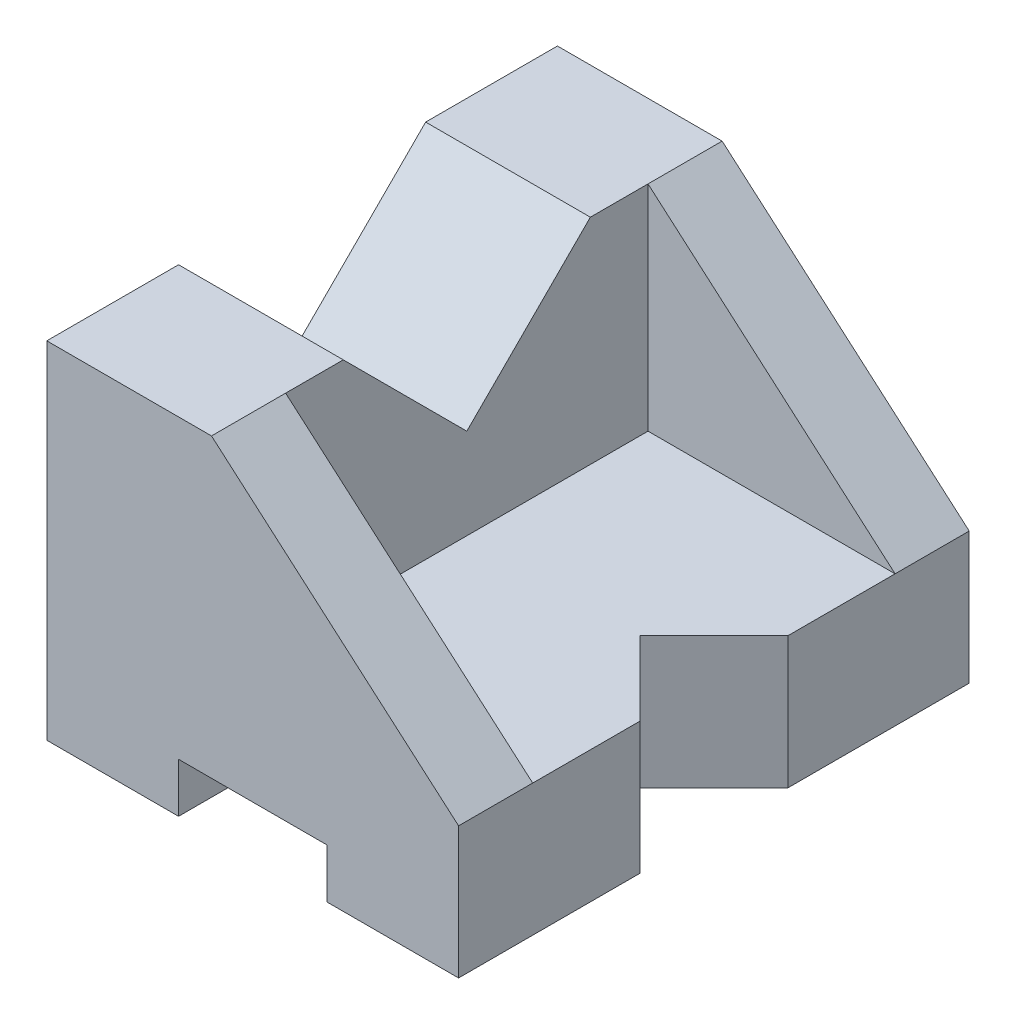
ISO-10303-21;
HEADER;
FILE_DESCRIPTION(('STEP AP214'),'2;1');
FILE_NAME('part.step','',(''),(''),'','','');
FILE_SCHEMA(('AUTOMOTIVE_DESIGN { 1 0 10303 214 1 1 1 1 }'));
ENDSEC;
DATA;
#1=APPLICATION_CONTEXT('core data for automotive mechanical design processes');
#2=APPLICATION_PROTOCOL_DEFINITION('international standard','automotive_design',2000,#1);
#3=PRODUCT_CONTEXT('',#1,'mechanical');
#4=PRODUCT('Part','Part','',(#3));
#5=PRODUCT_RELATED_PRODUCT_CATEGORY('part','',(#4));
#6=PRODUCT_DEFINITION_FORMATION('','',#4);
#7=PRODUCT_DEFINITION_CONTEXT('part definition',#1,'design');
#8=PRODUCT_DEFINITION('design','',#6,#7);
#9=PRODUCT_DEFINITION_SHAPE('','',#8);
#10=(LENGTH_UNIT() NAMED_UNIT(*) SI_UNIT(.MILLI.,.METRE.));
#11=(NAMED_UNIT(*) PLANE_ANGLE_UNIT() SI_UNIT($,.RADIAN.));
#12=(NAMED_UNIT(*) SI_UNIT($,.STERADIAN.) SOLID_ANGLE_UNIT());
#13=UNCERTAINTY_MEASURE_WITH_UNIT(LENGTH_MEASURE(1.E-05),#10,'distance_accuracy_value','');
#14=(GEOMETRIC_REPRESENTATION_CONTEXT(3) GLOBAL_UNCERTAINTY_ASSIGNED_CONTEXT((#13)) GLOBAL_UNIT_ASSIGNED_CONTEXT((#10,
#11,#12)) REPRESENTATION_CONTEXT('',''));
#15=CARTESIAN_POINT('',(0.,0.,0.));
#16=DIRECTION('',(0.,0.,1.));
#17=DIRECTION('',(1.,0.,0.));
#18=AXIS2_PLACEMENT_3D('',#15,#16,#17);
#19=CARTESIAN_POINT('',(-50.,0.,62.));
#20=DIRECTION('',(0.,1.,0.));
#21=DIRECTION('',(0.,0.,1.));
#22=AXIS2_PLACEMENT_3D('',#19,#20,#21);
#23=PLANE('',#22);
#24=DIRECTION('',(0.,0.,1.));
#25=VECTOR('',#24,1.);
#26=CARTESIAN_POINT('',(18.,0.,-62.001));
#27=LINE('',#26,#25);
#28=CARTESIAN_POINT('',(18.,0.,-62.));
#29=VERTEX_POINT('',#28);
#30=CARTESIAN_POINT('',(18.,0.,62.));
#31=VERTEX_POINT('',#30);
#32=EDGE_CURVE('E166',#29,#31,#27,.T.);
#33=ORIENTED_EDGE('',*,*,#32,.F.);
#34=DIRECTION('',(1.,0.,0.));
#35=VECTOR('',#34,1.);
#36=CARTESIAN_POINT('',(-50.,0.,-62.));
#37=LINE('',#36,#35);
#38=CARTESIAN_POINT('',(50.,0.,-62.));
#39=VERTEX_POINT('',#38);
#40=EDGE_CURVE('E190',#29,#39,#37,.T.);
#41=ORIENTED_EDGE('',*,*,#40,.T.);
#42=DIRECTION('',(0.,0.,-1.));
#43=VECTOR('',#42,1.);
#44=CARTESIAN_POINT('',(50.,0.,62.));
#45=LINE('',#44,#43);
#46=CARTESIAN_POINT('',(50.,0.,-18.));
#47=VERTEX_POINT('',#46);
#48=EDGE_CURVE('E216',#47,#39,#45,.T.);
#49=ORIENTED_EDGE('',*,*,#48,.F.);
#50=DIRECTION('',(0.707106781186548,0.,-0.707106781186547));
#51=VECTOR('',#50,1.);
#52=CARTESIAN_POINT('',(50.,0.,-18.));
#53=LINE('',#52,#51);
#54=CARTESIAN_POINT('',(32.,0.,0.));
#55=VERTEX_POINT('',#54);
#56=EDGE_CURVE('E297',#55,#47,#53,.T.);
#57=ORIENTED_EDGE('',*,*,#56,.F.);
#58=DIRECTION('',(-0.707106781186548,0.,-0.707106781186547));
#59=VECTOR('',#58,1.);
#60=CARTESIAN_POINT('',(32.,0.,0.));
#61=LINE('',#60,#59);
#62=CARTESIAN_POINT('',(50.,0.,18.));
#63=VERTEX_POINT('',#62);
#64=EDGE_CURVE('E312',#63,#55,#61,.T.);
#65=ORIENTED_EDGE('',*,*,#64,.F.);
#66=CARTESIAN_POINT('',(50.,0.,62.));
#67=VERTEX_POINT('',#66);
#68=EDGE_CURVE('E220',#67,#63,#45,.T.);
#69=ORIENTED_EDGE('',*,*,#68,.F.);
#70=DIRECTION('',(1.,0.,0.));
#71=VECTOR('',#70,1.);
#72=CARTESIAN_POINT('',(-50.,0.,62.));
#73=LINE('',#72,#71);
#74=EDGE_CURVE('E267',#31,#67,#73,.T.);
#75=ORIENTED_EDGE('',*,*,#74,.F.);
#76=EDGE_LOOP('',(#33,#41,#49,#57,#65,#69,#75));
#77=FACE_BOUND('',#76,.T.);
#78=ADVANCED_FACE('F39',(#77),#23,.F.);
#79=CARTESIAN_POINT('',(0.,0.,-62.));
#80=DIRECTION('',(0.,0.,1.));
#81=DIRECTION('',(1.,0.,0.));
#82=AXIS2_PLACEMENT_3D('',#79,#80,#81);
#83=PLANE('',#82);
#84=DIRECTION('',(0.,1.,0.));
#85=VECTOR('',#84,1.);
#86=CARTESIAN_POINT('',(-18.,0.,-62.));
#87=LINE('',#86,#85);
#88=CARTESIAN_POINT('',(-18.,0.,-62.));
#89=VERTEX_POINT('',#88);
#90=CARTESIAN_POINT('',(-18.,12.,-62.));
#91=VERTEX_POINT('',#90);
#92=EDGE_CURVE('E53',#89,#91,#87,.T.);
#93=ORIENTED_EDGE('',*,*,#92,.F.);
#94=CARTESIAN_POINT('',(-50.,0.,-62.));
#95=VERTEX_POINT('',#94);
#96=EDGE_CURVE('E177',#95,#89,#37,.T.);
#97=ORIENTED_EDGE('',*,*,#96,.F.);
#98=DIRECTION('',(0.,-1.,0.));
#99=VECTOR('',#98,1.);
#100=CARTESIAN_POINT('',(-50.,84.,-62.));
#101=LINE('',#100,#99);
#102=CARTESIAN_POINT('',(-50.,84.,-62.));
#103=VERTEX_POINT('',#102);
#104=EDGE_CURVE('E195',#103,#95,#101,.T.);
#105=ORIENTED_EDGE('',*,*,#104,.F.);
#106=DIRECTION('',(-1.,0.,0.));
#107=VECTOR('',#106,1.);
#108=CARTESIAN_POINT('',(-10.,84.,-62.));
#109=LINE('',#108,#107);
#110=CARTESIAN_POINT('',(-10.,84.,-62.));
#111=VERTEX_POINT('',#110);
#112=EDGE_CURVE('E196',#111,#103,#109,.T.);
#113=ORIENTED_EDGE('',*,*,#112,.F.);
#114=DIRECTION('',(-0.755689082789818,0.654930538417842,0.));
#115=VECTOR('',#114,1.);
#116=CARTESIAN_POINT('',(50.,32.,-62.));
#117=LINE('',#116,#115);
#118=CARTESIAN_POINT('',(50.,32.,-62.));
#119=VERTEX_POINT('',#118);
#120=EDGE_CURVE('E187',#119,#111,#117,.T.);
#121=ORIENTED_EDGE('',*,*,#120,.F.);
#122=DIRECTION('',(0.,1.,0.));
#123=VECTOR('',#122,1.);
#124=CARTESIAN_POINT('',(50.,0.,-62.));
#125=LINE('',#124,#123);
#126=EDGE_CURVE('E188',#39,#119,#125,.T.);
#127=ORIENTED_EDGE('',*,*,#126,.F.);
#128=ORIENTED_EDGE('',*,*,#40,.F.);
#129=DIRECTION('',(0.,-1.,0.));
#130=VECTOR('',#129,1.);
#131=CARTESIAN_POINT('',(18.,0.,-62.));
#132=LINE('',#131,#130);
#133=CARTESIAN_POINT('',(18.,12.,-62.));
#134=VERTEX_POINT('',#133);
#135=EDGE_CURVE('E305',#134,#29,#132,.T.);
#136=ORIENTED_EDGE('',*,*,#135,.F.);
#137=DIRECTION('',(1.,0.,0.));
#138=VECTOR('',#137,1.);
#139=CARTESIAN_POINT('',(-18.,12.,-62.));
#140=LINE('',#139,#138);
#141=EDGE_CURVE('E178',#91,#134,#140,.T.);
#142=ORIENTED_EDGE('',*,*,#141,.F.);
#143=EDGE_LOOP('',(#93,#97,#105,#113,#121,#127,#128,#136,#142));
#144=FACE_BOUND('',#143,.T.);
#145=ADVANCED_FACE('F174',(#144),#83,.F.);
#146=ORIENTED_EDGE('',*,*,#96,.T.);
#147=DIRECTION('',(0.,0.,1.));
#148=VECTOR('',#147,1.);
#149=CARTESIAN_POINT('',(-18.,0.,-62.001));
#150=LINE('',#149,#148);
#151=CARTESIAN_POINT('',(-18.,0.,62.));
#152=VERTEX_POINT('',#151);
#153=EDGE_CURVE('E165',#89,#152,#150,.T.);
#154=ORIENTED_EDGE('',*,*,#153,.T.);
#155=CARTESIAN_POINT('',(-50.,0.,62.));
#156=VERTEX_POINT('',#155);
#157=EDGE_CURVE('E269',#156,#152,#73,.T.);
#158=ORIENTED_EDGE('',*,*,#157,.F.);
#159=DIRECTION('',(0.,0.,-1.));
#160=VECTOR('',#159,1.);
#161=CARTESIAN_POINT('',(-50.,0.,62.));
#162=LINE('',#161,#160);
#163=EDGE_CURVE('E184',#156,#95,#162,.T.);
#164=ORIENTED_EDGE('',*,*,#163,.T.);
#165=EDGE_LOOP('',(#146,#154,#158,#164));
#166=FACE_BOUND('',#165,.T.);
#167=ADVANCED_FACE('F185',(#166),#23,.F.);
#168=CARTESIAN_POINT('',(50.,0.,62.));
#169=DIRECTION('',(-1.,0.,0.));
#170=DIRECTION('',(0.,0.,1.));
#171=AXIS2_PLACEMENT_3D('',#168,#169,#170);
#172=PLANE('',#171);
#173=DIRECTION('',(0.,1.,0.));
#174=VECTOR('',#173,1.);
#175=CARTESIAN_POINT('',(50.,-0.001000000000001,-18.));
#176=LINE('',#175,#174);
#177=CARTESIAN_POINT('',(50.,32.,-18.));
#178=VERTEX_POINT('',#177);
#179=EDGE_CURVE('E293',#47,#178,#176,.T.);
#180=ORIENTED_EDGE('',*,*,#179,.F.);
#181=ORIENTED_EDGE('',*,*,#48,.T.);
#182=ORIENTED_EDGE('',*,*,#126,.T.);
#183=DIRECTION('',(0.,0.,-1.));
#184=VECTOR('',#183,1.);
#185=CARTESIAN_POINT('',(50.,32.,62.));
#186=LINE('',#185,#184);
#187=CARTESIAN_POINT('',(50.,32.,-44.));
#188=VERTEX_POINT('',#187);
#189=EDGE_CURVE('E209',#188,#119,#186,.T.);
#190=ORIENTED_EDGE('',*,*,#189,.F.);
#191=DIRECTION('',(0.,0.,-1.));
#192=VECTOR('',#191,1.);
#193=CARTESIAN_POINT('',(50.,32.,-44.));
#194=LINE('',#193,#192);
#195=EDGE_CURVE('E258',#178,#188,#194,.T.);
#196=ORIENTED_EDGE('',*,*,#195,.F.);
#197=EDGE_LOOP('',(#180,#181,#182,#190,#196));
#198=FACE_BOUND('',#197,.T.);
#199=ADVANCED_FACE('F291',(#198),#172,.F.);
#200=CARTESIAN_POINT('',(-10.,84.,62.));
#201=DIRECTION('',(0.,-1.,0.));
#202=DIRECTION('',(0.,0.,-1.));
#203=AXIS2_PLACEMENT_3D('',#200,#201,#202);
#204=PLANE('',#203);
#205=DIRECTION('',(1.,0.,0.));
#206=VECTOR('',#205,1.);
#207=CARTESIAN_POINT('',(-134.,84.,30.));
#208=LINE('',#207,#206);
#209=CARTESIAN_POINT('',(-50.,84.,30.));
#210=VERTEX_POINT('',#209);
#211=CARTESIAN_POINT('',(-10.,84.,30.));
#212=VERTEX_POINT('',#211);
#213=EDGE_CURVE('E233',#210,#212,#208,.T.);
#214=ORIENTED_EDGE('',*,*,#213,.F.);
#215=DIRECTION('',(0.,0.,-1.));
#216=VECTOR('',#215,1.);
#217=CARTESIAN_POINT('',(-50.,84.,62.));
#218=LINE('',#217,#216);
#219=CARTESIAN_POINT('',(-50.,84.,62.));
#220=VERTEX_POINT('',#219);
#221=EDGE_CURVE('E205',#220,#210,#218,.T.);
#222=ORIENTED_EDGE('',*,*,#221,.F.);
#223=DIRECTION('',(-1.,0.,0.));
#224=VECTOR('',#223,1.);
#225=CARTESIAN_POINT('',(-10.,84.,62.));
#226=LINE('',#225,#224);
#227=CARTESIAN_POINT('',(-10.,84.,62.));
#228=VERTEX_POINT('',#227);
#229=EDGE_CURVE('E274',#228,#220,#226,.T.);
#230=ORIENTED_EDGE('',*,*,#229,.F.);
#231=DIRECTION('',(0.,0.,-1.));
#232=VECTOR('',#231,1.);
#233=CARTESIAN_POINT('',(-10.,84.,62.));
#234=LINE('',#233,#232);
#235=CARTESIAN_POINT('',(-10.,84.,44.));
#236=VERTEX_POINT('',#235);
#237=EDGE_CURVE('E210',#228,#236,#234,.T.);
#238=ORIENTED_EDGE('',*,*,#237,.T.);
#239=EDGE_CURVE('E211',#236,#212,#234,.T.);
#240=ORIENTED_EDGE('',*,*,#239,.T.);
#241=EDGE_LOOP('',(#214,#222,#230,#238,#240));
#242=FACE_BOUND('',#241,.T.);
#243=ADVANCED_FACE('F238',(#242),#204,.F.);
#244=CARTESIAN_POINT('',(50.,32.,62.));
#245=DIRECTION('',(-0.654930538417842,-0.755689082789818,0.));
#246=DIRECTION('',(0.755689082789818,-0.654930538417842,0.));
#247=AXIS2_PLACEMENT_3D('',#244,#245,#246);
#248=PLANE('',#247);
#249=DIRECTION('',(0.755689082789818,-0.654930538417842,0.));
#250=VECTOR('',#249,1.);
#251=CARTESIAN_POINT('',(50.,32.,44.));
#252=LINE('',#251,#250);
#253=CARTESIAN_POINT('',(50.,32.,44.));
#254=VERTEX_POINT('',#253);
#255=EDGE_CURVE('E221',#236,#254,#252,.T.);
#256=ORIENTED_EDGE('',*,*,#255,.F.);
#257=ORIENTED_EDGE('',*,*,#237,.F.);
#258=DIRECTION('',(-0.755689082789818,0.654930538417842,0.));
#259=VECTOR('',#258,1.);
#260=CARTESIAN_POINT('',(50.,32.,62.));
#261=LINE('',#260,#259);
#262=CARTESIAN_POINT('',(50.,32.,62.));
#263=VERTEX_POINT('',#262);
#264=EDGE_CURVE('E273',#263,#228,#261,.T.);
#265=ORIENTED_EDGE('',*,*,#264,.F.);
#266=EDGE_CURVE('E213',#263,#254,#186,.T.);
#267=ORIENTED_EDGE('',*,*,#266,.T.);
#268=EDGE_LOOP('',(#256,#257,#265,#267));
#269=FACE_BOUND('',#268,.T.);
#270=ADVANCED_FACE('F383',(#269),#248,.F.);
#271=DIRECTION('',(-0.755689082789818,0.654930538417842,0.));
#272=VECTOR('',#271,1.);
#273=CARTESIAN_POINT('',(50.,32.,-44.));
#274=LINE('',#273,#272);
#275=CARTESIAN_POINT('',(-10.,84.,-44.));
#276=VERTEX_POINT('',#275);
#277=EDGE_CURVE('E222',#188,#276,#274,.T.);
#278=ORIENTED_EDGE('',*,*,#277,.F.);
#279=ORIENTED_EDGE('',*,*,#189,.T.);
#280=ORIENTED_EDGE('',*,*,#120,.T.);
#281=EDGE_CURVE('E202',#276,#111,#234,.T.);
#282=ORIENTED_EDGE('',*,*,#281,.F.);
#283=EDGE_LOOP('',(#278,#279,#280,#282));
#284=FACE_BOUND('',#283,.T.);
#285=ADVANCED_FACE('F290',(#284),#248,.F.);
#286=CARTESIAN_POINT('',(-50.,84.,62.));
#287=DIRECTION('',(1.,0.,0.));
#288=DIRECTION('',(0.,1.,0.));
#289=AXIS2_PLACEMENT_3D('',#286,#287,#288);
#290=PLANE('',#289);
#291=DIRECTION('',(0.,-0.707106781186548,-0.707106781186548));
#292=VECTOR('',#291,1.);
#293=CARTESIAN_POINT('',(-50.,100.,46.));
#294=LINE('',#293,#292);
#295=CARTESIAN_POINT('',(-50.,54.,0.));
#296=VERTEX_POINT('',#295);
#297=EDGE_CURVE('E50',#210,#296,#294,.T.);
#298=ORIENTED_EDGE('',*,*,#297,.T.);
#299=DIRECTION('',(0.,0.707106781186548,-0.707106781186548));
#300=VECTOR('',#299,1.);
#301=CARTESIAN_POINT('',(-50.,38.,16.));
#302=LINE('',#301,#300);
#303=CARTESIAN_POINT('',(-50.,84.,-30.));
#304=VERTEX_POINT('',#303);
#305=EDGE_CURVE('E11',#296,#304,#302,.T.);
#306=ORIENTED_EDGE('',*,*,#305,.T.);
#307=EDGE_CURVE('E206',#304,#103,#218,.T.);
#308=ORIENTED_EDGE('',*,*,#307,.T.);
#309=ORIENTED_EDGE('',*,*,#104,.T.);
#310=ORIENTED_EDGE('',*,*,#163,.F.);
#311=DIRECTION('',(0.,-1.,0.));
#312=VECTOR('',#311,1.);
#313=CARTESIAN_POINT('',(-50.,84.,62.));
#314=LINE('',#313,#312);
#315=EDGE_CURVE('E203',#220,#156,#314,.T.);
#316=ORIENTED_EDGE('',*,*,#315,.F.);
#317=ORIENTED_EDGE('',*,*,#221,.T.);
#318=EDGE_LOOP('',(#298,#306,#308,#309,#310,#316,#317));
#319=FACE_BOUND('',#318,.T.);
#320=ADVANCED_FACE('F41',(#319),#290,.F.);
#321=ORIENTED_EDGE('',*,*,#68,.T.);
#322=DIRECTION('',(0.,1.,0.));
#323=VECTOR('',#322,1.);
#324=CARTESIAN_POINT('',(50.,-0.001000000000001,18.));
#325=LINE('',#324,#323);
#326=CARTESIAN_POINT('',(50.,32.,18.));
#327=VERTEX_POINT('',#326);
#328=EDGE_CURVE('E322',#63,#327,#325,.T.);
#329=ORIENTED_EDGE('',*,*,#328,.T.);
#330=EDGE_CURVE('E260',#254,#327,#194,.T.);
#331=ORIENTED_EDGE('',*,*,#330,.F.);
#332=ORIENTED_EDGE('',*,*,#266,.F.);
#333=DIRECTION('',(0.,1.,0.));
#334=VECTOR('',#333,1.);
#335=CARTESIAN_POINT('',(50.,0.,62.));
#336=LINE('',#335,#334);
#337=EDGE_CURVE('E275',#67,#263,#336,.T.);
#338=ORIENTED_EDGE('',*,*,#337,.F.);
#339=EDGE_LOOP('',(#321,#329,#331,#332,#338));
#340=FACE_BOUND('',#339,.T.);
#341=ADVANCED_FACE('F346',(#340),#172,.F.);
#342=ORIENTED_EDGE('',*,*,#307,.F.);
#343=DIRECTION('',(1.,0.,0.));
#344=VECTOR('',#343,1.);
#345=CARTESIAN_POINT('',(-134.,84.,-30.));
#346=LINE('',#345,#344);
#347=CARTESIAN_POINT('',(-10.,84.,-30.));
#348=VERTEX_POINT('',#347);
#349=EDGE_CURVE('E244',#304,#348,#346,.T.);
#350=ORIENTED_EDGE('',*,*,#349,.T.);
#351=EDGE_CURVE('E215',#348,#276,#234,.T.);
#352=ORIENTED_EDGE('',*,*,#351,.T.);
#353=ORIENTED_EDGE('',*,*,#281,.T.);
#354=ORIENTED_EDGE('',*,*,#112,.T.);
#355=EDGE_LOOP('',(#342,#350,#352,#353,#354));
#356=FACE_BOUND('',#355,.T.);
#357=ADVANCED_FACE('F278',(#356),#204,.F.);
#358=CARTESIAN_POINT('',(0.,0.,62.));
#359=DIRECTION('',(0.,0.,1.));
#360=DIRECTION('',(1.,0.,0.));
#361=AXIS2_PLACEMENT_3D('',#358,#359,#360);
#362=PLANE('',#361);
#363=DIRECTION('',(0.,-1.,0.));
#364=VECTOR('',#363,1.);
#365=CARTESIAN_POINT('',(-18.,0.,62.));
#366=LINE('',#365,#364);
#367=CARTESIAN_POINT('',(-18.,12.,62.));
#368=VERTEX_POINT('',#367);
#369=EDGE_CURVE('E164',#368,#152,#366,.T.);
#370=ORIENTED_EDGE('',*,*,#369,.F.);
#371=DIRECTION('',(-1.,0.,0.));
#372=VECTOR('',#371,1.);
#373=CARTESIAN_POINT('',(-18.,12.,62.));
#374=LINE('',#373,#372);
#375=CARTESIAN_POINT('',(18.,12.,62.));
#376=VERTEX_POINT('',#375);
#377=EDGE_CURVE('E168',#376,#368,#374,.T.);
#378=ORIENTED_EDGE('',*,*,#377,.F.);
#379=DIRECTION('',(0.,1.,0.));
#380=VECTOR('',#379,1.);
#381=CARTESIAN_POINT('',(18.,0.,62.));
#382=LINE('',#381,#380);
#383=EDGE_CURVE('E306',#31,#376,#382,.T.);
#384=ORIENTED_EDGE('',*,*,#383,.F.);
#385=ORIENTED_EDGE('',*,*,#74,.T.);
#386=ORIENTED_EDGE('',*,*,#337,.T.);
#387=ORIENTED_EDGE('',*,*,#264,.T.);
#388=ORIENTED_EDGE('',*,*,#229,.T.);
#389=ORIENTED_EDGE('',*,*,#315,.T.);
#390=ORIENTED_EDGE('',*,*,#157,.T.);
#391=EDGE_LOOP('',(#370,#378,#384,#385,#386,#387,#388,#389,#390));
#392=FACE_BOUND('',#391,.T.);
#393=ADVANCED_FACE('F351',(#392),#362,.T.);
#394=CARTESIAN_POINT('',(-10.,156.,44.));
#395=DIRECTION('',(0.,0.,-1.));
#396=DIRECTION('',(-1.,0.,0.));
#397=AXIS2_PLACEMENT_3D('',#394,#395,#396);
#398=PLANE('',#397);
#399=ORIENTED_EDGE('',*,*,#255,.T.);
#400=DIRECTION('',(1.,0.,0.));
#401=VECTOR('',#400,1.);
#402=CARTESIAN_POINT('',(-10.,32.,44.));
#403=LINE('',#402,#401);
#404=CARTESIAN_POINT('',(-10.,32.,44.));
#405=VERTEX_POINT('',#404);
#406=EDGE_CURVE('E251',#405,#254,#403,.T.);
#407=ORIENTED_EDGE('',*,*,#406,.F.);
#408=DIRECTION('',(0.,-1.,0.));
#409=VECTOR('',#408,1.);
#410=CARTESIAN_POINT('',(-10.,156.,44.));
#411=LINE('',#410,#409);
#412=EDGE_CURVE('E264',#236,#405,#411,.T.);
#413=ORIENTED_EDGE('',*,*,#412,.F.);
#414=EDGE_LOOP('',(#399,#407,#413));
#415=FACE_BOUND('',#414,.T.);
#416=ADVANCED_FACE('F405',(#415),#398,.T.);
#417=CARTESIAN_POINT('',(-10.,156.,-44.));
#418=DIRECTION('',(0.,0.,1.));
#419=DIRECTION('',(1.,0.,0.));
#420=AXIS2_PLACEMENT_3D('',#417,#418,#419);
#421=PLANE('',#420);
#422=ORIENTED_EDGE('',*,*,#277,.T.);
#423=DIRECTION('',(0.,-1.,0.));
#424=VECTOR('',#423,1.);
#425=CARTESIAN_POINT('',(-10.,156.,-44.));
#426=LINE('',#425,#424);
#427=CARTESIAN_POINT('',(-10.,32.,-44.));
#428=VERTEX_POINT('',#427);
#429=EDGE_CURVE('E263',#276,#428,#426,.T.);
#430=ORIENTED_EDGE('',*,*,#429,.T.);
#431=DIRECTION('',(-1.,0.,0.));
#432=VECTOR('',#431,1.);
#433=CARTESIAN_POINT('',(-10.,32.,-44.));
#434=LINE('',#433,#432);
#435=EDGE_CURVE('E257',#188,#428,#434,.T.);
#436=ORIENTED_EDGE('',*,*,#435,.F.);
#437=EDGE_LOOP('',(#422,#430,#436));
#438=FACE_BOUND('',#437,.T.);
#439=ADVANCED_FACE('F337',(#438),#421,.T.);
#440=CARTESIAN_POINT('',(-10.,156.,-44.));
#441=DIRECTION('',(1.,0.,0.));
#442=DIRECTION('',(0.,0.,-1.));
#443=AXIS2_PLACEMENT_3D('',#440,#441,#442);
#444=PLANE('',#443);
#445=DIRECTION('',(0.,-0.707106781186547,-0.707106781186547));
#446=VECTOR('',#445,1.);
#447=CARTESIAN_POINT('',(-10.,54.,0.));
#448=LINE('',#447,#446);
#449=CARTESIAN_POINT('',(-10.,54.,0.));
#450=VERTEX_POINT('',#449);
#451=EDGE_CURVE('E247',#212,#450,#448,.T.);
#452=ORIENTED_EDGE('',*,*,#451,.F.);
#453=ORIENTED_EDGE('',*,*,#239,.F.);
#454=ORIENTED_EDGE('',*,*,#412,.T.);
#455=DIRECTION('',(0.,0.,1.));
#456=VECTOR('',#455,1.);
#457=CARTESIAN_POINT('',(-10.,32.,-44.));
#458=LINE('',#457,#456);
#459=EDGE_CURVE('E248',#428,#405,#458,.T.);
#460=ORIENTED_EDGE('',*,*,#459,.F.);
#461=ORIENTED_EDGE('',*,*,#429,.F.);
#462=ORIENTED_EDGE('',*,*,#351,.F.);
#463=DIRECTION('',(0.,0.707106781186547,-0.707106781186547));
#464=VECTOR('',#463,1.);
#465=CARTESIAN_POINT('',(-10.,84.,-30.));
#466=LINE('',#465,#464);
#467=EDGE_CURVE('E245',#450,#348,#466,.T.);
#468=ORIENTED_EDGE('',*,*,#467,.F.);
#469=EDGE_LOOP('',(#452,#453,#454,#460,#461,#462,#468));
#470=FACE_BOUND('',#469,.T.);
#471=ADVANCED_FACE('F338',(#470),#444,.T.);
#472=CARTESIAN_POINT('',(0.,32.,0.));
#473=DIRECTION('',(0.,1.,0.));
#474=DIRECTION('',(0.,0.,1.));
#475=AXIS2_PLACEMENT_3D('',#472,#473,#474);
#476=PLANE('',#475);
#477=DIRECTION('',(-0.707106781186548,0.,0.707106781186547));
#478=VECTOR('',#477,1.);
#479=CARTESIAN_POINT('',(50.,32.,-18.));
#480=LINE('',#479,#478);
#481=CARTESIAN_POINT('',(32.,32.,0.));
#482=VERTEX_POINT('',#481);
#483=EDGE_CURVE('E65',#178,#482,#480,.T.);
#484=ORIENTED_EDGE('',*,*,#483,.F.);
#485=ORIENTED_EDGE('',*,*,#195,.T.);
#486=ORIENTED_EDGE('',*,*,#435,.T.);
#487=ORIENTED_EDGE('',*,*,#459,.T.);
#488=ORIENTED_EDGE('',*,*,#406,.T.);
#489=ORIENTED_EDGE('',*,*,#330,.T.);
#490=DIRECTION('',(0.707106781186548,0.,0.707106781186547));
#491=VECTOR('',#490,1.);
#492=CARTESIAN_POINT('',(32.,32.,0.));
#493=LINE('',#492,#491);
#494=EDGE_CURVE('E325',#482,#327,#493,.T.);
#495=ORIENTED_EDGE('',*,*,#494,.F.);
#496=EDGE_LOOP('',(#484,#485,#486,#487,#488,#489,#495));
#497=FACE_BOUND('',#496,.T.);
#498=ADVANCED_FACE('F345',(#497),#476,.T.);
#499=CARTESIAN_POINT('',(-134.,84.,-30.));
#500=DIRECTION('',(0.,-0.707106781186548,-0.707106781186548));
#501=DIRECTION('',(0.,0.707106781186548,-0.707106781186548));
#502=AXIS2_PLACEMENT_3D('',#499,#500,#501);
#503=PLANE('',#502);
#504=DIRECTION('',(1.,0.,0.));
#505=VECTOR('',#504,1.);
#506=CARTESIAN_POINT('',(-134.,54.,0.));
#507=LINE('',#506,#505);
#508=EDGE_CURVE('E240',#296,#450,#507,.T.);
#509=ORIENTED_EDGE('',*,*,#508,.T.);
#510=ORIENTED_EDGE('',*,*,#467,.T.);
#511=ORIENTED_EDGE('',*,*,#349,.F.);
#512=ORIENTED_EDGE('',*,*,#305,.F.);
#513=EDGE_LOOP('',(#509,#510,#511,#512));
#514=FACE_BOUND('',#513,.T.);
#515=ADVANCED_FACE('F407',(#514),#503,.F.);
#516=CARTESIAN_POINT('',(-134.,54.,0.));
#517=DIRECTION('',(0.,-0.707106781186548,0.707106781186548));
#518=DIRECTION('',(0.,-0.707106781186548,-0.707106781186548));
#519=AXIS2_PLACEMENT_3D('',#516,#517,#518);
#520=PLANE('',#519);
#521=ORIENTED_EDGE('',*,*,#213,.T.);
#522=ORIENTED_EDGE('',*,*,#451,.T.);
#523=ORIENTED_EDGE('',*,*,#508,.F.);
#524=ORIENTED_EDGE('',*,*,#297,.F.);
#525=EDGE_LOOP('',(#521,#522,#523,#524));
#526=FACE_BOUND('',#525,.T.);
#527=ADVANCED_FACE('F234',(#526),#520,.F.);
#528=CARTESIAN_POINT('',(32.,-0.001000000000001,0.));
#529=DIRECTION('',(-0.707106781186548,0.,0.707106781186548));
#530=DIRECTION('',(0.707106781186548,0.,0.707106781186547));
#531=AXIS2_PLACEMENT_3D('',#528,#529,#530);
#532=PLANE('',#531);
#533=ORIENTED_EDGE('',*,*,#64,.T.);
#534=DIRECTION('',(0.,1.,0.));
#535=VECTOR('',#534,1.);
#536=CARTESIAN_POINT('',(32.,-0.001000000000001,0.));
#537=LINE('',#536,#535);
#538=EDGE_CURVE('E330',#55,#482,#537,.T.);
#539=ORIENTED_EDGE('',*,*,#538,.T.);
#540=ORIENTED_EDGE('',*,*,#494,.T.);
#541=ORIENTED_EDGE('',*,*,#328,.F.);
#542=EDGE_LOOP('',(#533,#539,#540,#541));
#543=FACE_BOUND('',#542,.T.);
#544=ADVANCED_FACE('F347',(#543),#532,.F.);
#545=CARTESIAN_POINT('',(50.,-0.001000000000001,-18.));
#546=DIRECTION('',(-0.707106781186548,0.,-0.707106781186548));
#547=DIRECTION('',(-0.707106781186548,0.,0.707106781186547));
#548=AXIS2_PLACEMENT_3D('',#545,#546,#547);
#549=PLANE('',#548);
#550=ORIENTED_EDGE('',*,*,#56,.T.);
#551=ORIENTED_EDGE('',*,*,#179,.T.);
#552=ORIENTED_EDGE('',*,*,#483,.T.);
#553=ORIENTED_EDGE('',*,*,#538,.F.);
#554=EDGE_LOOP('',(#550,#551,#552,#553));
#555=FACE_BOUND('',#554,.T.);
#556=ADVANCED_FACE('F364',(#555),#549,.F.);
#557=CARTESIAN_POINT('',(-18.,0.,-62.001));
#558=DIRECTION('',(-1.,0.,0.));
#559=DIRECTION('',(0.,0.,1.));
#560=AXIS2_PLACEMENT_3D('',#557,#558,#559);
#561=PLANE('',#560);
#562=ORIENTED_EDGE('',*,*,#92,.T.);
#563=DIRECTION('',(0.,0.,1.));
#564=VECTOR('',#563,1.);
#565=CARTESIAN_POINT('',(-18.,12.,-62.001));
#566=LINE('',#565,#564);
#567=EDGE_CURVE('E311',#91,#368,#566,.T.);
#568=ORIENTED_EDGE('',*,*,#567,.T.);
#569=ORIENTED_EDGE('',*,*,#369,.T.);
#570=ORIENTED_EDGE('',*,*,#153,.F.);
#571=EDGE_LOOP('',(#562,#568,#569,#570));
#572=FACE_BOUND('',#571,.T.);
#573=ADVANCED_FACE('F162',(#572),#561,.F.);
#574=CARTESIAN_POINT('',(-18.,12.,-62.001));
#575=DIRECTION('',(0.,1.,0.));
#576=DIRECTION('',(0.,0.,1.));
#577=AXIS2_PLACEMENT_3D('',#574,#575,#576);
#578=PLANE('',#577);
#579=ORIENTED_EDGE('',*,*,#141,.T.);
#580=DIRECTION('',(0.,0.,1.));
#581=VECTOR('',#580,1.);
#582=CARTESIAN_POINT('',(18.,12.,-62.001));
#583=LINE('',#582,#581);
#584=EDGE_CURVE('E316',#134,#376,#583,.T.);
#585=ORIENTED_EDGE('',*,*,#584,.T.);
#586=ORIENTED_EDGE('',*,*,#377,.T.);
#587=ORIENTED_EDGE('',*,*,#567,.F.);
#588=EDGE_LOOP('',(#579,#585,#586,#587));
#589=FACE_BOUND('',#588,.T.);
#590=ADVANCED_FACE('F360',(#589),#578,.F.);
#591=CARTESIAN_POINT('',(18.,0.,-62.001));
#592=DIRECTION('',(1.,0.,0.));
#593=DIRECTION('',(0.,0.,-1.));
#594=AXIS2_PLACEMENT_3D('',#591,#592,#593);
#595=PLANE('',#594);
#596=ORIENTED_EDGE('',*,*,#135,.T.);
#597=ORIENTED_EDGE('',*,*,#32,.T.);
#598=ORIENTED_EDGE('',*,*,#383,.T.);
#599=ORIENTED_EDGE('',*,*,#584,.F.);
#600=EDGE_LOOP('',(#596,#597,#598,#599));
#601=FACE_BOUND('',#600,.T.);
#602=ADVANCED_FACE('F352',(#601),#595,.F.);
#603=CLOSED_SHELL('',(#78,#145,#167,#199,#243,#270,#285,#320,#341,#357,#393,#416,#439,#471,#498,
#515,#527,#544,#556,#573,#590,#602));
#604=MANIFOLD_SOLID_BREP('B2',#603);
#605=ADVANCED_BREP_SHAPE_REPRESENTATION('',(#18,#604),#14);
#606=SHAPE_DEFINITION_REPRESENTATION(#9,#605);
ENDSEC;
END-ISO-10303-21;
